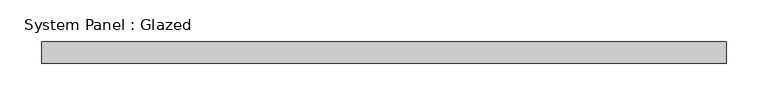
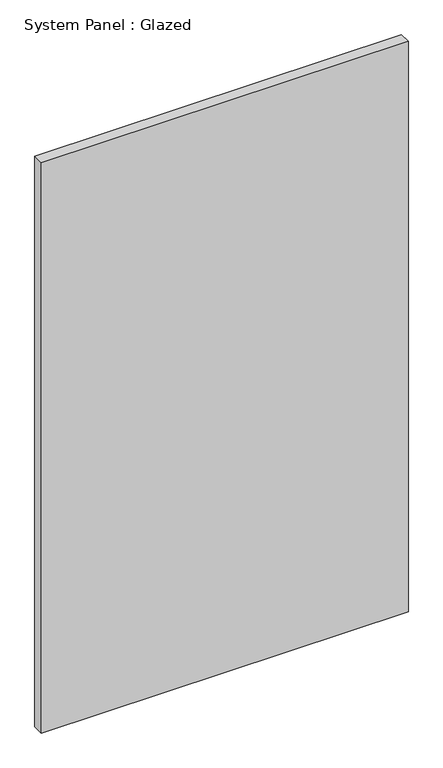
"""IFC4 building model written with IfcOpenShell, lengths in millimetres: plate geometry, System Panel : Glazed."""

from ifc_helpers import new_model, si_unit, origin, origin_with_axes, place, context, project, spatial, polyline, outline, extrude, source, transform, mapped, element, save


def system_panel_glazed_37765a37(model_context):
    return source(origin(), model_context, "Body", "SweptSolid", [
        extrude(outline(polyline([(409.575, 19.05), (-409.575, 19.05), (-409.575, 44.45), (409.575, 44.45), (409.575, 19.05)])), origin_with_axes(), (0.0, 0.0, 1.0), 1344.9817095),
    ])


if __name__ == "__main__":
    model = new_model("IFC4")
    model_context = context("Model", 3, world=origin())
    ifc_project = project(units=[si_unit("LENGTHUNIT", "METRE", prefix="MILLI")], contexts=[model_context])
    site = spatial("IfcSite", under=ifc_project)
    building = spatial("IfcBuilding", under=site)
    placement = place(None, origin())
    system_panel_glazed_shape = system_panel_glazed_37765a37(model_context)
    element("IfcPlate", 1, ObjectType="System Panel : Glazed", at=placement, inside=building, context=model_context, shape_type="MappedRepresentation", body=[
        mapped(system_panel_glazed_shape, transform((0.0, 0.0, 0.0), x_axis=(1.0, 0.0, 0.0), y_axis=(0.0, 1.0, 0.0), z_axis=(0.0, 0.0, 1.0))),
    ])
    save(model, "model.ifc")

# Revit data of these elements
# Type "System Panel : Glazed"
#   Construction Type Id = "GSP4R"
#   Analytic Construction = "1/8 in Pilkington single glazing"
#   Visual Light Transmittance = 0.9
#   Solar Heat Gain Coefficient = 0.86
#   Heat Transfer Coefficient (U) = 1.18115 BTU/(h·ft²·°F)
#   Define Thermal Properties by = 1
# Element 1 (IfcPlate, "System Panel : Glazed")
#   Materials on its faces: "Glass"
# Materials
#   "Glass": class "Glass", colour RGB 0 128 192, transparency 0.75, Description = "Soda Lime Glass", Cost = 0
